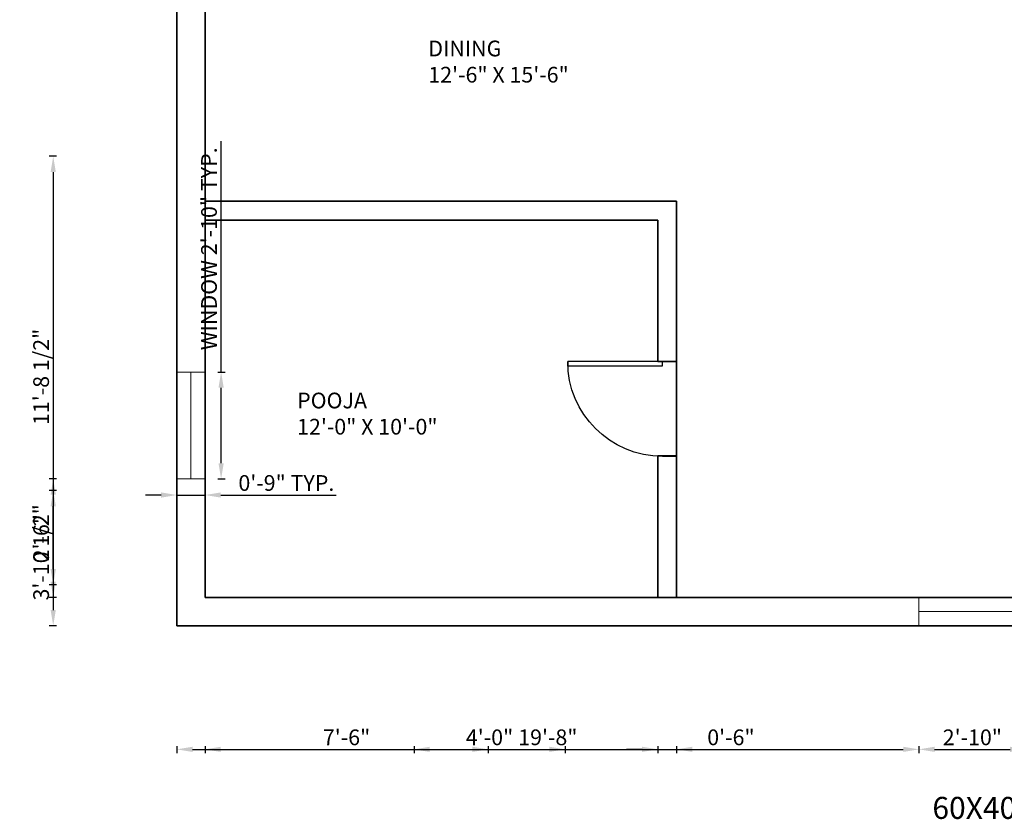
# Model space of a CAD drawing. Units: inches. Extents: x -48 to 817, y -530 to 78.
# Tile 1 of 7: x -48 to 266, y -530 to -276. Entities that reach past the tile are written whole.
import ezdxf

# ---------------------------------------------------------------- set-up
doc = ezdxf.new("R2010")
doc.units = ezdxf.units.IN
for name, color, linetype, lineweight in [('A-ANNO-DIMS', 2, 'Continuous', 18), ('A-AREA-IDEN', 7, 'Continuous', 18), ('A-DOOR', 3, 'Continuous', 25), ('A-GLAZ', 4, 'Continuous', 18), ('A-WALL', 7, 'Continuous', 35), ('txt', 7, 'Continuous', 18)]:
    doc.layers.add(name, color=color, linetype=linetype, lineweight=lineweight)
doc.styles.get("Standard").update_dxf_attribs({"font": 'arial.ttf'})
doc.dimstyles.new('ISO-25', dxfattribs={"dimtxt": 5, "dimasz": 5, "dimexe": 1.25, "dimexo": 0.625, "dimtad": 1, "dimlunit": 3, "dimtxsty": 'Standard', "dimcen": 2.5, "dimadec": 0, "dimazin": 0, "dimtfac": 1, "dimtmove": 0, "dimatfit": 3, "dimfxl": 1, "dimfxlon": 1, "dimarcsym": 0})

# ---------------------------------------------------------------- blocks, each defined once
blk = doc.blocks.new('*U2')
for p, q in [((0, 0), (0, -6)), ((40, 0), (40, -6))]:
    blk.add_line(p, q)
blk.add_lwpolyline([(0, 0), (0, 40), (1.75, 40), (1.75, 0)], close=True)
blk.add_arc((0, 0), 40, 0, 90)
blk = doc.blocks.new('WIN-34IN')
blk.add_line((4.5, 34), (4.5, 0))
blk.add_lwpolyline([(9, 34), (0, 34), (0, 0), (9, 0)], close=True)
blk = doc.blocks.new('*D22')
at = {"layer": 'A-ANNO-DIMS', "color": 0, "lineweight": -2, "transparency": 16777216}
for p, q in [((16.53, -387.62), (16.53, -314.21)), ((15.53, -387.62), (17.78, -387.62)), ((16.53, -416.62), (16.53, -392.62)), ((15.53, -421.62), (17.78, -421.62))]:
    blk.add_line(p, q, dxfattribs=at)
at = {"layer": 'A-ANNO-DIMS', "color": 0, "transparency": 16777216}
for points in [[(15.69, -392.62), (17.36, -392.62), (16.53, -387.62)], [(15.69, -416.62), (17.36, -416.62), (16.53, -421.62)]]:
    blk.add_solid(points, dxfattribs=at)
at = {"layer": 'Defpoints', "color": 0, "transparency": 16777216}
for p in [(11.43, -387.62), (16.53, -387.62), (11.43, -421.62)]:
    blk.add_point(p, dxfattribs=at)
at = {"layer": 'A-ANNO-DIMS', "color": 0, "transparency": 16777216, "insert": (13.32, -348.42), "char_height": 5, "attachment_point": 5, "rotation": 90}
blk.add_mtext('WINDOW 2\'-10" TYP.', dxfattribs=at)
blk = doc.blocks.new('*D23')
at = {"layer": 'A-ANNO-DIMS', "color": 0, "lineweight": -2, "transparency": 16777216}
for p, q in [((2.43, -425.72), (2.43, -427.97)), ((11.43, -425.72), (11.43, -427.97)), ((-2.57, -426.72), (-7.57, -426.72)), ((2.43, -426.72), (11.43, -426.72)), ((16.43, -426.72), (53.15, -426.72))]:
    blk.add_line(p, q, dxfattribs=at)
at = {"layer": 'A-ANNO-DIMS', "color": 0, "transparency": 16777216}
for points in [[(-2.57, -425.89), (-2.57, -427.55), (2.43, -426.72)], [(16.43, -425.89), (16.43, -427.55), (11.43, -426.72)]]:
    blk.add_solid(points, dxfattribs=at)
at = {"layer": 'Defpoints', "color": 0, "transparency": 16777216}
for p in [(2.43, -421.62), (11.43, -421.62), (11.43, -426.72)]:
    blk.add_point(p, dxfattribs=at)
at = {"layer": 'A-ANNO-DIMS', "color": 0, "transparency": 16777216, "insert": (37.29, -423.54), "char_height": 5, "attachment_point": 5}
blk.add_mtext('0\'-9" TYP.', dxfattribs=at)
blk = doc.blocks.new('*D52')
at = {"layer": 'A-ANNO-DIMS', "color": 0, "lineweight": -2, "transparency": 16777216}
for p, q in [((-35.87, -421.62), (-38.12, -421.62)), ((-36.87, -426.62), (-36.87, -463.28)), ((-35.87, -468.28), (-38.12, -468.28))]:
    blk.add_line(p, q, dxfattribs=at)
at = {"layer": 'A-ANNO-DIMS', "color": 0, "transparency": 16777216}
for points in [[(-37.71, -426.62), (-36.04, -426.62), (-36.87, -421.62)], [(-37.71, -463.28), (-36.04, -463.28), (-36.87, -468.28)]]:
    blk.add_solid(points, dxfattribs=at)
at = {"layer": 'Defpoints', "color": 0, "transparency": 16777216}
for p in [(2.43, -421.62), (-36.87, -468.28), (2.43, -468.28)]:
    blk.add_point(p, dxfattribs=at)
at = {"layer": 'A-ANNO-DIMS', "color": 0, "transparency": 16777216, "insert": (-40.08, -444.95), "char_height": 5, "attachment_point": 5, "rotation": 90}
blk.add_mtext('3\'-10 1/2"', dxfattribs=at)
blk = doc.blocks.new('*D56')
at = {"layer": 'A-ANNO-DIMS', "color": 0, "lineweight": -2, "transparency": 16777216}
for p, q in [((2.43, -506.59), (2.43, -508.84)), ((238.5, -506.59), (238.5, -508.84)), ((7.43, -507.59), (233.5, -507.59))]:
    blk.add_line(p, q, dxfattribs=at)
at = {"layer": 'A-ANNO-DIMS', "color": 0, "transparency": 16777216}
for points in [[(7.43, -506.76), (7.43, -508.42), (2.43, -507.59)], [(233.5, -506.76), (233.5, -508.42), (238.5, -507.59)]]:
    blk.add_solid(points, dxfattribs=at)
at = {"layer": 'Defpoints', "color": 0, "transparency": 16777216}
for p in [(2.43, -468.28), (238.5, -468.28), (238.5, -507.59)]:
    blk.add_point(p, dxfattribs=at)
at = {"layer": 'A-ANNO-DIMS', "color": 0, "transparency": 16777216, "insert": (120.46, -504.41), "char_height": 5, "attachment_point": 5}
blk.add_mtext('19\'-8"', dxfattribs=at)
blk = doc.blocks.new('*D59')
at = {"layer": 'A-ANNO-DIMS', "color": 0, "lineweight": -2, "transparency": 16777216}
for p, q in [((155.43, -506.59), (155.43, -508.84)), ((161.43, -506.59), (161.43, -508.84)), ((150.43, -507.59), (145.43, -507.59)), ((155.43, -507.59), (161.43, -507.59)), ((166.43, -507.59), (185.97, -507.59))]:
    blk.add_line(p, q, dxfattribs=at)
at = {"layer": 'A-ANNO-DIMS', "color": 0, "transparency": 16777216}
for points in [[(150.43, -506.76), (150.43, -508.42), (155.43, -507.59)], [(166.43, -506.76), (166.43, -508.42), (161.43, -507.59)]]:
    blk.add_solid(points, dxfattribs=at)
at = {"layer": 'Defpoints', "color": 0, "transparency": 16777216}
for p in [(155.43, -141.28), (161.43, -147.28), (161.43, -507.59)]:
    blk.add_point(p, dxfattribs=at)
at = {"layer": 'A-ANNO-DIMS', "color": 0, "transparency": 16777216, "insert": (178.7, -504.41), "char_height": 5, "attachment_point": 5}
blk.add_mtext('0\'-6"', dxfattribs=at)
blk = doc.blocks.new('*D65')
at = {"layer": 'A-ANNO-DIMS', "color": 0, "lineweight": -2, "transparency": 16777216}
for p, q in [((811.62, -384.28), (813.87, -384.28)), ((812.62, -389.28), (812.62, -409.4)), ((811.62, -414.4), (813.87, -414.4))]:
    blk.add_line(p, q, dxfattribs=at)
at = {"layer": 'A-ANNO-DIMS', "color": 0, "transparency": 16777216}
for points in [[(811.79, -389.28), (813.45, -389.28), (812.62, -384.28)], [(811.79, -409.4), (813.45, -409.4), (812.62, -414.4)]]:
    blk.add_solid(points, dxfattribs=at)
at = {"layer": 'Defpoints', "color": 0, "transparency": 16777216}
for p in [(161.43, -384.28), (161.43, -414.4), (812.62, -414.4)]:
    blk.add_point(p, dxfattribs=at)
at = {"layer": 'A-ANNO-DIMS', "color": 0, "transparency": 16777216, "insert": (809.44, -399.34), "char_height": 5, "attachment_point": 5, "rotation": 90}
blk.add_mtext('2\'-6"', dxfattribs=at)
blk = doc.blocks.new('*D66')
at = {"layer": 'A-ANNO-DIMS', "color": 0, "lineweight": -2, "transparency": 16777216}
for p, q in [((811.62, -414.4), (813.87, -414.4)), ((812.62, -419.4), (812.62, -454.28)), ((811.62, -459.28), (813.87, -459.28))]:
    blk.add_line(p, q, dxfattribs=at)
at = {"layer": 'A-ANNO-DIMS', "color": 0, "transparency": 16777216}
for points in [[(811.79, -419.4), (813.45, -419.4), (812.62, -414.4)], [(811.79, -454.28), (813.45, -454.28), (812.62, -459.28)]]:
    blk.add_solid(points, dxfattribs=at)
at = {"layer": 'Defpoints', "color": 0, "transparency": 16777216}
for p in [(161.43, -414.4), (161.43, -459.28), (812.62, -459.28)]:
    blk.add_point(p, dxfattribs=at)
at = {"layer": 'A-ANNO-DIMS', "color": 0, "transparency": 16777216, "insert": (809.44, -436.84), "char_height": 5, "attachment_point": 5, "rotation": 90}
blk.add_mtext('3\'-9"', dxfattribs=at)
blk = doc.blocks.new('*D70')
at = {"layer": 'A-ANNO-DIMS', "color": 0, "lineweight": -2, "transparency": 16777216}
for p, q in [((-35.87, -319.02), (-38.12, -319.02)), ((-36.87, -324.02), (-36.87, -454.28)), ((-35.87, -459.28), (-38.12, -459.28))]:
    blk.add_line(p, q, dxfattribs=at)
at = {"layer": 'A-ANNO-DIMS', "color": 0, "transparency": 16777216}
for points in [[(-37.71, -324.02), (-36.04, -324.02), (-36.87, -319.02)], [(-37.71, -454.28), (-36.04, -454.28), (-36.87, -459.28)]]:
    blk.add_solid(points, dxfattribs=at)
at = {"layer": 'Defpoints', "color": 0, "transparency": 16777216}
for p in [(479.43, -319.02), (-36.87, -459.28), (479.43, -459.28)]:
    blk.add_point(p, dxfattribs=at)
at = {"layer": 'A-ANNO-DIMS', "color": 0, "transparency": 16777216, "insert": (-40.08, -389.15), "char_height": 5, "attachment_point": 5, "rotation": 90}
blk.add_mtext('11\'-8 1/2"', dxfattribs=at)
blk = doc.blocks.new('*D71')
at = {"layer": 'A-ANNO-DIMS', "color": 0, "lineweight": -2, "transparency": 16777216}
for p, q in [((11.43, -506.59), (11.43, -508.84)), ((101.43, -506.59), (101.43, -508.84)), ((16.43, -507.59), (96.43, -507.59))]:
    blk.add_line(p, q, dxfattribs=at)
at = {"layer": 'A-ANNO-DIMS', "color": 0, "transparency": 16777216}
for points in [[(16.43, -506.76), (16.43, -508.42), (11.43, -507.59)], [(96.43, -506.76), (96.43, -508.42), (101.43, -507.59)]]:
    blk.add_solid(points, dxfattribs=at)
at = {"layer": 'Defpoints', "color": 0, "transparency": 16777216}
for p in [(11.43, 2.72), (101.43, 2.72), (101.43, -507.59)]:
    blk.add_point(p, dxfattribs=at)
at = {"layer": 'A-ANNO-DIMS', "color": 0, "transparency": 16777216, "insert": (56.43, -504.41), "char_height": 5, "attachment_point": 5}
blk.add_mtext('7\'-6"', dxfattribs=at)
blk = doc.blocks.new('*D77')
at = {"layer": 'A-ANNO-DIMS', "color": 0, "lineweight": -2, "transparency": 16777216}
for p, q in [((77.91, -506.59), (77.91, -508.84)), ((125.92, -506.59), (125.92, -508.84)), ((82.91, -507.59), (120.92, -507.59))]:
    blk.add_line(p, q, dxfattribs=at)
at = {"layer": 'A-ANNO-DIMS', "color": 0, "transparency": 16777216}
for points in [[(82.91, -506.76), (82.91, -508.42), (77.91, -507.59)], [(120.92, -506.76), (120.92, -508.42), (125.92, -507.59)]]:
    blk.add_solid(points, dxfattribs=at)
at = {"layer": 'Defpoints', "color": 0, "transparency": 16777216}
for p in [(77.91, -256.74), (125.92, -256.74), (125.92, -507.59)]:
    blk.add_point(p, dxfattribs=at)
at = {"layer": 'A-ANNO-DIMS', "color": 0, "transparency": 16777216, "insert": (101.92, -504.41), "char_height": 5, "attachment_point": 5}
blk.add_mtext('4\'-0"', dxfattribs=at)
blk = doc.blocks.new('*D84')
at = {"layer": 'A-ANNO-DIMS', "color": 0, "lineweight": -2, "transparency": 16777216}
for p, q in [((-35.87, -425.28), (-38.12, -425.28)), ((-36.87, -450.28), (-36.87, -430.28)), ((-35.87, -455.28), (-38.12, -455.28))]:
    blk.add_line(p, q, dxfattribs=at)
at = {"layer": 'A-ANNO-DIMS', "color": 0, "transparency": 16777216}
for points in [[(-37.71, -430.28), (-36.04, -430.28), (-36.87, -425.28)], [(-37.71, -450.28), (-36.04, -450.28), (-36.87, -455.28)]]:
    blk.add_solid(points, dxfattribs=at)
at = {"layer": 'Defpoints', "color": 0, "transparency": 16777216}
for p in [(-36.87, -425.28), (623.43, -425.28), (623.43, -455.28)]:
    blk.add_point(p, dxfattribs=at)
at = {"layer": 'A-ANNO-DIMS', "color": 0, "transparency": 16777216, "insert": (-40.05, -440.28), "char_height": 5, "attachment_point": 5, "rotation": 90}
blk.add_mtext('2\'-6"', dxfattribs=at)
blk = doc.blocks.new('*D85')
at = {"layer": 'A-ANNO-DIMS', "color": 0, "lineweight": -2, "transparency": 16777216}
for p, q in [((238.5, -506.59), (238.5, -508.84)), ((272.5, -506.59), (272.5, -508.84)), ((243.5, -507.59), (267.5, -507.59))]:
    blk.add_line(p, q, dxfattribs=at)
at = {"layer": 'A-ANNO-DIMS', "color": 0, "transparency": 16777216}
for points in [[(243.5, -506.76), (243.5, -508.42), (238.5, -507.59)], [(267.5, -506.76), (267.5, -508.42), (272.5, -507.59)]]:
    blk.add_solid(points, dxfattribs=at)
at = {"layer": 'Defpoints', "color": 0, "transparency": 16777216}
for p in [(238.5, -468.28), (272.5, -468.28), (272.5, -507.59)]:
    blk.add_point(p, dxfattribs=at)
at = {"layer": 'A-ANNO-DIMS', "color": 0, "transparency": 16777216, "insert": (255.5, -504.41), "char_height": 5, "attachment_point": 5}
blk.add_mtext('2\'-10"', dxfattribs=at)

msp = doc.modelspace()

# ---------------------------------------------------------------- linework, layer by layer
at = {"layer": 'A-GLAZ'}
for p, q in [((238.498, -459.275), (238.498, -468.275)), ((272.498, -463.775), (238.498, -463.775))]:
    msp.add_line(p, q, dxfattribs=at)
at = {"layer": 'A-WALL'}
for p, q in [((2.427, -468.275), (2.427, 11.725)), ((11.427, -459.275), (11.427, -257.275)), ((11.427, -333.275), (155.427, -333.275)), ((155.427, -333.275), (161.427, -333.275)), ((161.427, -333.275), (161.427, -459.275)), ((11.427, -339.275), (155.427, -339.275)), ((155.427, -339.275), (155.427, -384.275)), ((155.427, -384.275), (161.427, -384.275)), ((155.427, -414.275), (161.427, -414.275)), ((155.427, -414.275), (155.427, -459.275)), ((273.233, -459.275), (11.427, -459.275)), ((722.427, -468.275), (2.427, -468.275))]:
    msp.add_line(p, q, dxfattribs=at)

# ---------------------------------------------------------------- block references
at = {"layer": 'A-DOOR', "xscale": -0.753026279444749, "yscale": 0.753026279444749, "zscale": 0.753026279444749, "rotation": 90}
msp.add_blockref('*U2', (156.909, -384.275), dxfattribs=at)
at = {"layer": 'A-GLAZ'}
msp.add_blockref('WIN-34IN', (2.427, -421.62), dxfattribs=at)

# ---------------------------------------------------------------- texts
at = {"layer": 'A-AREA-IDEN', "char_height": 5, "attachment_point": 1}
for s, width, insert in [('DINING\\P12\'-6" X 15\'-6"', 69.24966, (82.439, -282.227)), ('POOJA\\P12\'-0" X 10\'-0"', 70.85294, (40.699, -394.158))]:
    msp.add_mtext_dynamic_manual_height_columns(s, width=width, gutter_width=12.5, heights=[0], dxfattribs=dict(at, insert=insert))
at = {"layer": 'txt', "insert": (242.785, -522.709), "char_height": 7, "attachment_point": 1}
msp.add_mtext_dynamic_manual_height_columns('60X40 SOUTH FACING HOUSE PLAN', width=437.74312, gutter_width=12.5, heights=[0], dxfattribs=at)

# ---------------------------------------------------------------- dimensions: what is measured, and where the dimension line sits
at = {"layer": 'A-ANNO-DIMS'}
for base, p1, p2, picture, middle in [((101.427, -507.589), (11.427, 2.725), (101.427, 2.725), '*D71', (56.427, -504.411)), ((161.427, -507.589), (155.427, -141.275), (161.427, -147.275), '*D59', (178.698, -504.411)), ((125.924, -507.589), (77.913, -256.743), (125.924, -256.743), '*D77', (101.919, -504.411)), ((238.498, -507.589), (2.427, -468.275), (238.498, -468.275), '*D56', (120.463, -504.411)), ((272.498, -507.589), (238.498, -468.275), (272.498, -468.275), '*D85', (255.498, -504.411))]:
    dim = msp.add_linear_dim(base=base, p1=p1, p2=p2, dimstyle='ISO-25', override={"dimdec": 1, "dimlfac": 1, "dimrnd": 0, "dimzin": 1, "dimdsep": 46, "dimlunit": 4, "dimfrac": 2}, dxfattribs=at)
    dim.commit()
    dim.dimension.update_dxf_attribs({"geometry": picture, "text_midpoint": middle})
dim = msp.add_linear_dim(base=(16.527, -387.62), p1=(11.427, -421.62), p2=(11.427, -387.62), angle=90, text='WINDOW <> TYP.', dimstyle='ISO-25', override={"dimdec": 1, "dimlfac": 1, "dimrnd": 0, "dimzin": 1, "dimdsep": 46, "dimlunit": 4, "dimfrac": 2}, dxfattribs=at)
dim.commit()
dim.dimension.update_dxf_attribs({"geometry": '*D22', "text_midpoint": (13.315, -348.417)})
for base, p1, p2, picture, middle in [((-36.873, -459.275), (479.427, -319.021), (479.427, -459.275), '*D70', (-40.083, -389.148)), ((812.622, -414.396), (161.427, -384.275), (161.427, -414.396), '*D65', (809.444, -399.336)), ((812.622, -459.275), (161.427, -414.396), (161.427, -459.275), '*D66', (809.442, -436.836)), ((-36.873, -468.275), (2.427, -421.62), (2.427, -468.275), '*D52', (-40.085, -444.948)), ((-36.873, -425.275), (623.427, -455.275), (623.427, -425.275), '*D84', (-40.051, -440.275))]:
    dim = msp.add_linear_dim(base=base, p1=p1, p2=p2, angle=90, dimstyle='ISO-25', override={"dimdec": 1, "dimlfac": 1, "dimrnd": 0, "dimzin": 1, "dimdsep": 46, "dimlunit": 4, "dimfrac": 2}, dxfattribs=at)
    dim.commit()
    dim.dimension.update_dxf_attribs({"geometry": picture, "text_midpoint": middle})
dim = msp.add_linear_dim(base=(11.427, -426.72), p1=(2.427, -421.62), p2=(11.427, -421.62), text='<> TYP.', dimstyle='ISO-25', override={"dimdec": 1, "dimlfac": 1, "dimrnd": 0, "dimzin": 1, "dimdsep": 46, "dimlunit": 4, "dimfrac": 2}, dxfattribs=at)
dim.commit()
dim.dimension.update_dxf_attribs({"geometry": '*D23', "text_midpoint": (37.291, -423.542)})

doc.saveas('drawing.dxf')
